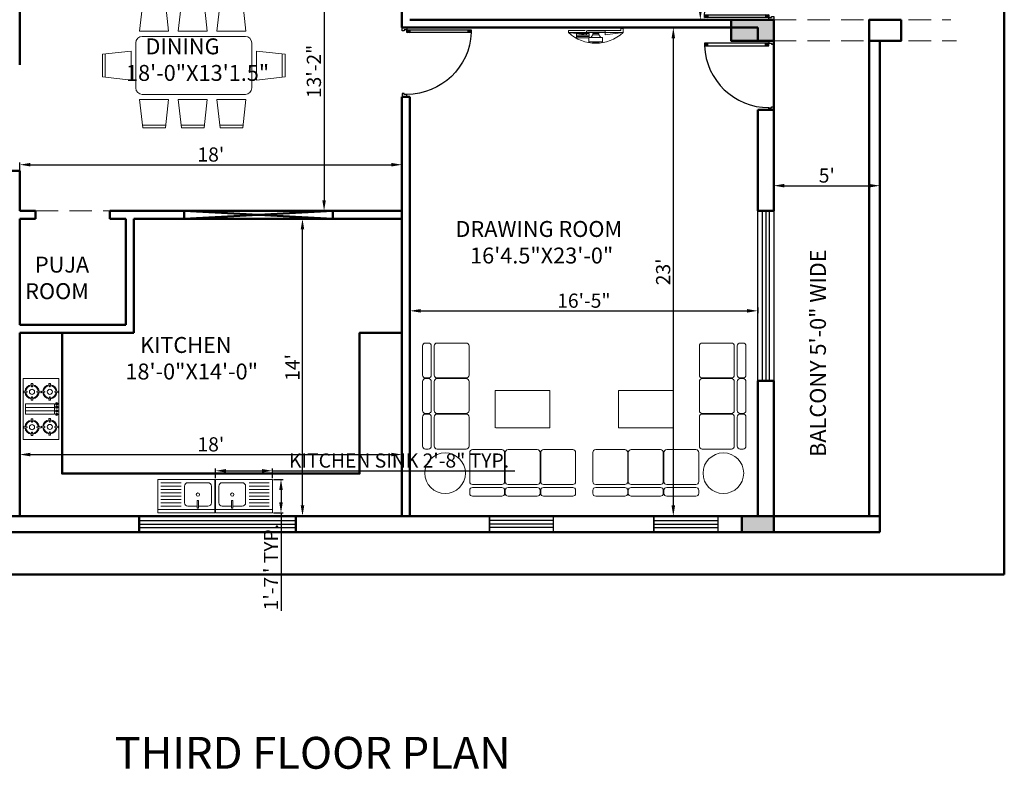
# Model space of a CAD drawing. Units: millimetres. Extents: x 1706 to 5913, y 156 to 1716.
# Tile 11 of 26: x 3523 to 4080, y 219 to 642. Entities that reach past the tile are written whole.
import ezdxf

# ---------------------------------------------------------------- set-up
doc = ezdxf.new("R2010")
doc.units = ezdxf.units.MM
doc.linetypes.add('DASHED', pattern=[19.05, 12.7, -6.35])
for name, color, linetype, lineweight in [('A-ANNO-DIMS', 2, 'Continuous', 18), ('A-ANNO-TEXT', 7, 'Continuous', 18), ('A-AREA-IDEN', 3, 'Continuous', 18), ('A-COLS', 20, 'Continuous', 50), ('A-DOOR', 4, 'Continuous', 25), ('A-FLOR-OVHD', 9, 'DASHED', 18), ('A-FURN', 8, 'Continuous', 18), ('A-GLAZ', 150, 'Continuous', 25), ('A-WALL', 7, 'Continuous', 50)]:
    doc.layers.add(name, color=color, linetype=linetype, lineweight=lineweight)
doc.styles.get("Standard").update_dxf_attribs({"font": 'arial.ttf'})
doc.dimstyles.new('ISO-25', dxfattribs={"dimtxt": 8, "dimasz": 6, "dimexe": 1.25, "dimexo": 0.625, "dimtad": 1, "dimdec": 0, "dimlunit": 3, "dimtxsty": 'Standard', "dimcen": 2.5, "dimadec": 0, "dimazin": 0, "dimtfac": 1, "dimtdec": 0, "dimtmove": 0, "dimatfit": 3, "dimfxl": 1, "dimarcsym": 0})

# ---------------------------------------------------------------- blocks, each defined once
blk = doc.blocks.new('Puerta 01')
for p, q in [((-0.775, -0.026), (-0.737, -0.058)), ((-0.775, -0.058), (-0.737, -0.026)), ((-0.737, -0.058), (-0.737, -0.026)), ((-0.028, -0.058), (-0.066, -0.026)), ((-0.028, -0.026), (-0.066, -0.058)), ((-0.066, -0.058), (-0.066, -0.026))]:
    blk.add_line(p, q)
for points in [[(-0.028, 0), (-0.028, -0.026), (0.004, -0.026), (0.004, -0.036), (0.028, -0.036), (0.028, 0)], [(-0.028, -0.026), (-0.775, -0.026), (-0.775, -0.058), (-0.028, -0.058)], [(0.004, -0.774), (0.004, -0.764), (0.028, -0.764), (0.028, -0.8), (-0.028, -0.8), (-0.028, -0.774)]]:
    blk.add_lwpolyline(points, close=True)
blk.add_arc((-0.028, -0.026), 0.747, 182.4545, 270)
blk = doc.blocks.new('A$C57CF26DA')
for p, q in [((0, 0), (0, 420)), ((720, 420), (0, 420)), ((167, 413), (147, 413)), ((147, 413), (152, 373)), ((152, 373), (162, 373)), ((162, 373), (167, 413)), ((300, 391), (300, 49)), ((300, 391), (420, 391)), ((340, 391), (340, 49)), ((380, 391), (380, 49)), ((420, 391), (420, 49)), ((584, 413), (564, 413)), ((564, 413), (569, 373)), ((569, 373), (579, 373)), ((579, 373), (584, 413)), ((720, 0), (720, 420)), ((99, 320), (59, 325)), ((59, 325), (59, 305)), ((59, 305), (99, 310)), ((99, 310), (99, 320)), ((152, 257), (147, 217)), ((162, 257), (152, 257)), ((167, 217), (162, 257)), ((255, 325), (215, 320)), ((215, 320), (215, 310)), ((215, 310), (255, 305)), ((255, 305), (255, 325)), ((516, 320), (476, 325)), ((476, 325), (476, 305)), ((476, 305), (516, 310)), ((516, 310), (516, 320)), ((569, 257), (564, 217)), ((579, 257), (569, 257)), ((584, 217), (579, 257)), ((672, 325), (632, 320)), ((632, 320), (632, 310)), ((632, 310), (672, 305)), ((672, 305), (672, 325)), ((147, 217), (167, 217)), ((167, 203), (147, 203)), ((147, 203), (152, 163)), ((152, 163), (162, 163)), ((162, 163), (167, 203)), ((581, 203), (561, 203)), ((561, 203), (566, 163)), ((564, 217), (584, 217)), ((566, 163), (576, 163)), ((576, 163), (581, 203)), ((99, 110), (59, 115)), ((59, 115), (59, 95)), ((59, 95), (99, 100)), ((99, 100), (99, 110)), ((152, 47), (147, 7)), ((147, 7), (167, 7)), ((162, 47), (152, 47)), ((167, 7), (162, 47)), ((255, 115), (215, 110)), ((215, 110), (215, 100)), ((215, 100), (255, 95)), ((255, 95), (255, 115)), ((302, 39), (295, 39)), ((295, 39), (295, 11)), ((295, 11), (302, 11)), ((420, 49), (300, 49)), ((302, 11), (302, 39)), ((341, 39), (334, 39)), ((334, 39), (334, 11)), ((334, 11), (341, 11)), ((341, 11), (341, 39)), ((380, 11), (380, 39)), ((380, 39), (386, 39)), ((386, 11), (380, 11)), ((386, 39), (386, 11)), ((419, 11), (419, 39)), ((419, 39), (426, 39)), ((426, 11), (419, 11)), ((426, 39), (426, 11)), ((513, 110), (473, 115)), ((473, 115), (473, 95)), ((473, 95), (513, 100)), ((513, 100), (513, 110)), ((566, 47), (561, 7)), ((561, 7), (581, 7)), ((576, 47), (566, 47)), ((581, 7), (576, 47)), ((669, 115), (629, 110)), ((629, 110), (629, 100)), ((629, 100), (669, 95)), ((669, 95), (669, 115)), ((720, 0), (0, 0))]:
    blk.add_line(p, q)
for centre in [(157, 315), (574, 315), (157, 105), (571, 105)]:
    blk.add_circle(centre, 30)
for centre, radius, start, end in [((157, 315), 83, 95.5849, 174.4151), ((157, 315), 73, 95.3738, 174.6262), ((157, 315), 73, 5.3738, 84.6262), ((157, 315), 83, 5.5849, 84.4151), ((574, 315), 83, 95.5849, 174.4151), ((574, 315), 73, 95.3738, 174.6262), ((574, 315), 73, 5.3738, 84.6262), ((574, 315), 83, 5.5849, 84.4151), ((157, 315), 83, 185.5849, 264.4151), ((157, 315), 73, 185.3738, 264.6262), ((157, 315), 73, 275.3738, 354.6262), ((157, 315), 83, 275.5849, 354.4151), ((574, 315), 83, 185.5849, 264.4151), ((574, 315), 73, 185.3738, 264.6262), ((574, 315), 73, 275.3738, 354.6262), ((574, 315), 83, 275.5849, 354.4151), ((157, 105), 83, 95.5849, 174.4151), ((157, 105), 73, 95.3738, 174.6262), ((157, 105), 73, 5.3738, 84.6262), ((157, 105), 83, 5.5849, 84.4151), ((571, 105), 83, 95.5849, 174.4151), ((571, 105), 73, 95.3738, 174.6262), ((571, 105), 73, 5.3738, 84.6262), ((571, 105), 83, 5.5849, 84.4151), ((157, 105), 83, 185.5849, 264.4151), ((157, 105), 73, 185.3738, 264.6262), ((157, 105), 73, 275.3738, 354.6262), ((157, 105), 83, 275.5849, 354.4151), ((298, 25), 13.7, 104.4775, 255.5225), ((298, 25), 13.7, 284.4775, 75.5225), ((337, 25), 13.7, 104.4775, 255.5225), ((337, 25), 13.7, 284.4775, 75.5225), ((383, 25), 13.7, 104.4775, 255.5225), ((383, 25), 13.7, 284.4775, 75.5225), ((422, 25), 13.7, 104.4775, 255.5225), ((422, 25), 13.7, 284.4775, 75.5225), ((571, 105), 83, 185.5849, 264.4151), ((571, 105), 73, 185.3738, 264.6262), ((571, 105), 73, 275.3738, 354.6262), ((571, 105), 83, 275.5849, 354.4151)]:
    blk.add_arc(centre, radius, start, end)
blk = doc.blocks.new('A$C3404121D')
for p, q in [((0, 0), (0, 500)), ((0, 500), (850, 500)), ((0, 450), (850, 450)), ((850, 500), (850, 0)), ((50, 100), (50, 350)), ((100, 400), (240, 400)), ((240, 431), (240, 425)), ((260, 431), (240, 431)), ((240, 425), (240, 315)), ((240, 315), (260, 315)), ((260, 431), (260, 315)), ((260, 400), (400, 400)), ((450, 100), (450, 350)), ((502, 400), (801, 400)), ((502, 350), (801, 350)), ((502, 300), (801, 300)), ((502, 250), (801, 250)), ((502, 200), (801, 200)), ((502, 150), (801, 150)), ((850, 0), (0, 0)), ((400, 50), (100, 50)), ((502, 100), (801, 100)), ((801, 50), (502, 50))]:
    blk.add_line(p, q)
blk.add_circle((250, 228), 25)
for centre, start, end in [((100, 350), 90, 180), ((400, 350), 0, 90), ((100, 100), 180, 270), ((400, 100), 270, 0)]:
    blk.add_arc(centre, 50, start, end)
blk = doc.blocks.new('A$C59D7588A')
for p, q in [((0.575, 1.5), (0.623, 1.943)), ((0.618, 1.9), (0.982, 1.9)), ((0.623, 1.943), (0.978, 1.943)), ((0.978, 1.943), (1.025, 1.5)), ((1.175, 1.5), (1.223, 1.943)), ((1.218, 1.9), (1.582, 1.9)), ((1.223, 1.943), (1.578, 1.943)), ((1.578, 1.943), (1.625, 1.5)), ((1.775, 1.5), (1.823, 1.943)), ((1.818, 1.9), (2.182, 1.9)), ((1.823, 1.943), (2.178, 1.943)), ((2.178, 1.943), (2.225, 1.5)), ((1.025, 1.5), (0.575, 1.5)), ((0.616, 1.421), (2.216, 1.421)), ((1.625, 1.5), (1.175, 1.5)), ((2.225, 1.5), (1.775, 1.5)), ((0.516, 0.621), (0.516, 1.321)), ((2.316, 1.321), (2.316, 0.621)), ((0, 1.146), (0.443, 1.194)), ((0, 0.792), (0, 1.146)), ((0.043, 0.787), (0.043, 1.151)), ((0.443, 1.194), (0.443, 0.744)), ((2.832, 1.146), (2.389, 1.194)), ((2.389, 1.194), (2.389, 0.744)), ((2.789, 0.787), (2.789, 1.151)), ((2.832, 0.792), (2.832, 1.146)), ((0.443, 0.744), (0, 0.792)), ((2.389, 0.744), (2.832, 0.792)), ((2.216, 0.521), (0.616, 0.521)), ((1.025, 0.443), (0.575, 0.443)), ((0.575, 0.443), (0.623, 0)), ((0.978, 0), (1.025, 0.443)), ((1.625, 0.443), (1.175, 0.443)), ((1.175, 0.443), (1.223, 0)), ((1.578, 0), (1.625, 0.443)), ((2.225, 0.443), (1.775, 0.443)), ((1.775, 0.443), (1.823, 0)), ((2.178, 0), (2.225, 0.443)), ((0.618, 0.043), (0.982, 0.043)), ((1.218, 0.043), (1.582, 0.043)), ((1.818, 0.043), (2.182, 0.043)), ((0.623, 0), (0.978, 0)), ((1.223, 0), (1.578, 0)), ((1.823, 0), (2.178, 0))]:
    blk.add_line(p, q)
for centre, start, end in [((0.616, 1.321), 90, 180), ((2.216, 1.321), 0, 90), ((0.616, 0.621), 180, 270), ((2.216, 0.621), 270, 0)]:
    blk.add_arc(centre, 0.1, start, end)
blk = doc.blocks.new('A$C753D6792')
at = {"linetype": 'ByBlock'}
for p, q in [((0, 2530), (0, 2580)), ((50, 2630), (550, 2630)), ((600, 2580), (600, 2530)), ((610, 2530), (610, 2580)), ((660, 2630), (1160, 2630)), ((1210, 2580), (1210, 2530)), ((1220, 2530), (1220, 2580)), ((1270, 2630), (1770, 2630)), ((1820, 2580), (1820, 2530)), ((0, 1880), (0, 2380)), ((550, 2480), (50, 2480)), ((550, 2430), (50, 2430)), ((600, 2380), (600, 1880)), ((610, 1880), (610, 2380)), ((1160, 2480), (660, 2480)), ((1160, 2430), (660, 2430)), ((1210, 2380), (1210, 1880)), ((1220, 1880), (1220, 2380)), ((1770, 2480), (1270, 2480)), ((1770, 2430), (1270, 2430)), ((1820, 1880), (1820, 2380)), ((50, 1830), (427, 1830)), ((387, 1830), (550, 1830)), ((660, 1830), (1037, 1830)), ((997, 1830), (1160, 1830)), ((1270, 1830), (1647, 1830)), ((1607, 1830), (1770, 1830)), ((1830, 1770), (1830, 1393)), ((1880, 1820), (2380, 1820)), ((2430, 1270), (2430, 1770)), ((2480, 1270), (2480, 1770)), ((2530, 1820), (2580, 1820)), ((2630, 1770), (2630, 1270)), ((442, 815), (442, 1455)), ((442, 1455), (1372, 1455)), ((1382, 1455), (1382, 815)), ((1830, 1433), (1830, 1270)), ((2380, 1220), (1880, 1220)), ((1880, 1210), (2380, 1210)), ((2580, 1220), (2530, 1220)), ((2530, 1210), (2580, 1210)), ((1830, 1160), (1830, 783)), ((2430, 660), (2430, 1160)), ((2480, 660), (2480, 1160)), ((2630, 1160), (2630, 660)), ((1382, 815), (442, 815)), ((1830, 823), (1830, 660)), ((1830, 550), (1830, 173)), ((2380, 610), (1880, 610)), ((1880, 600), (2380, 600)), ((2430, 50), (2430, 550)), ((2480, 50), (2480, 550)), ((2580, 610), (2530, 610)), ((2530, 600), (2580, 600)), ((2630, 550), (2630, 50)), ((1830, 213), (1830, 50)), ((2380, 0), (1880, 0)), ((2580, 0), (2530, 0))]:
    blk.add_line(p, q, dxfattribs=at)
blk.add_circle((2242, 2235), 349, dxfattribs=at)
for centre, start, end in [((50, 2580), 90, 180), ((550, 2580), 0, 90), ((550, 2580), 0, 90), ((660, 2580), 90, 180), ((1160, 2580), 0, 90), ((1160, 2580), 0, 90), ((1270, 2580), 90, 180), ((1770, 2580), 0, 90), ((1770, 2580), 0, 90), ((50, 2530), 180, 270), ((50, 2380), 90, 180), ((550, 2530), 270, 0), ((550, 2530), 270, 0), ((550, 2380), 0, 90), ((550, 2380), 0, 90), ((660, 2530), 180, 270), ((660, 2380), 90, 180), ((1160, 2530), 270, 0), ((1160, 2530), 270, 0), ((1160, 2380), 0, 90), ((1160, 2380), 0, 90), ((1270, 2530), 180, 270), ((1270, 2380), 90, 180), ((1770, 2530), 270, 0), ((1770, 2530), 270, 0), ((1770, 2380), 0, 90), ((1770, 2380), 0, 90), ((50, 1880), 180, 270), ((550, 1880), 270, 0), ((660, 1880), 180, 270), ((1160, 1880), 270, 0), ((1270, 1880), 180, 270), ((1770, 1880), 270, 0), ((1880, 1770), 90, 180), ((2380, 1770), 0, 90), ((2530, 1770), 90, 180), ((2580, 1770), 0, 90), ((1880, 1270), 180, 270), ((1880, 1160), 90, 180), ((2380, 1270), 270, 0), ((2380, 1270), 270, 0), ((2380, 1160), 0, 90), ((2530, 1270), 180, 270), ((2530, 1270), 180, 270), ((2530, 1160), 90, 180), ((2580, 1270), 270, 0), ((2580, 1270), 270, 0), ((2580, 1160), 0, 90), ((1880, 660), 180, 270), ((1880, 550), 90, 180), ((2380, 660), 270, 0), ((2380, 660), 270, 0), ((2380, 550), 0, 90), ((2530, 660), 180, 270), ((2530, 660), 180, 270), ((2530, 550), 90, 180), ((2580, 660), 270, 0), ((2580, 660), 270, 0), ((2580, 550), 0, 90), ((1880, 50), 180, 270), ((2380, 50), 270, 0), ((2380, 50), 270, 0), ((2530, 50), 180, 270), ((2530, 50), 180, 270), ((2580, 50), 270, 0), ((2580, 50), 270, 0)]:
    blk.add_arc(centre, 50, start, end, dxfattribs=at)
blk = doc.blocks.new('tv unit')
for p, q in [((4607, 2403), (5207, 2403)), ((4607, 2203), (4607, 2403)), ((5853, 2588), (5205, 2588)), ((5205, 2392), (5205, 2588)), ((5853, 2392), (5205, 2392)), ((5207, 2403), (5207, 2203)), ((5293, 2392), (5385, 2268)), ((5765, 2392), (5672, 2268)), ((5853, 2392), (5853, 2588)), ((5079, 2257), (4229, 2157)), ((6829, 2157), (4229, 2157)), ((4229, 2157), (4229, 2057)), ((5029, 2057), (4229, 2057)), ((4607, 2337), (5207, 2337)), ((4607, 2269), (5207, 2269)), ((5207, 2203), (4607, 2203)), ((5079, 2077), (5079, 2257)), ((5979, 2077), (5079, 2077)), ((6729, 2057), (5129, 2057)), ((5385, 2268), (5672, 2268)), ((5385, 2268), (5385, 2204)), ((5385, 2204), (5672, 2204)), ((5672, 2268), (5672, 2204)), ((5979, 2257), (6829, 2157)), ((5979, 2077), (5979, 2257)), ((6729, 2057), (6729, 1957)), ((6829, 1957), (6729, 1957)), ((6829, 2157), (6829, 1957))]:
    blk.add_line(p, q)
for points in [[(6829, 2157, 0.386509), (4229, 2157, -2.260033)], [(4242, 2140, -0.414214), (4270, 2168), (4561, 2168)]]:
    blk.add_lwpolyline(points, format="xyb")
blk.add_arc((5529, 609), 2006, 80.6925, 99.3075)
blk = doc.blocks.new('*D159')
at = {"layer": 'A-ANNO-DIMS', "color": 0, "lineweight": -2, "transparency": 16777216}
for p, q in [((3907.19, 843.39), (3906.51, 843.39)), ((3907.76, 837.39), (3907.76, 648.39)), ((3907.19, 642.39), (3906.51, 642.39))]:
    blk.add_line(p, q, dxfattribs=at)
at = {"layer": 'A-ANNO-DIMS', "color": 0, "transparency": 16777216}
for points in [[(3906.76, 837.39), (3908.76, 837.39), (3907.76, 843.39)], [(3906.76, 648.39), (3908.76, 648.39), (3907.76, 642.39)]]:
    blk.add_solid(points, dxfattribs=at)
at = {"layer": 'Defpoints', "color": 0, "transparency": 16777216}
for p in [(3907.82, 843.39), (3907.76, 642.39), (3907.82, 642.39)]:
    blk.add_point(p, dxfattribs=at)
at = {"layer": 'A-ANNO-DIMS', "color": 0, "transparency": 16777216, "insert": (3903.05, 742.89), "char_height": 8, "attachment_point": 5, "rotation": 90}
blk.add_mtext('16\'-9"', dxfattribs=at)
blk = doc.blocks.new('*D161')
at = {"layer": 'A-ANNO-DIMS', "color": 0, "lineweight": -2, "transparency": 16777216}
for p, q in [((3692.59, 691.89), (3696.44, 691.89)), ((3695.19, 685.89), (3695.19, 540.39)), ((3692.59, 534.39), (3696.44, 534.39))]:
    blk.add_line(p, q, dxfattribs=at)
at = {"layer": 'A-ANNO-DIMS', "color": 0, "transparency": 16777216}
for points in [[(3694.19, 685.89), (3696.19, 685.89), (3695.19, 691.89)], [(3694.19, 540.39), (3696.19, 540.39), (3695.19, 534.39)]]:
    blk.add_solid(points, dxfattribs=at)
at = {"layer": 'Defpoints', "color": 0, "transparency": 16777216}
for p in [(3691.96, 691.89), (3691.96, 534.39), (3695.19, 534.39)]:
    blk.add_point(p, dxfattribs=at)
at = {"layer": 'A-ANNO-DIMS', "color": 0, "transparency": 16777216, "insert": (3690.48, 613.14), "char_height": 8, "attachment_point": 5, "rotation": 90}
blk.add_mtext('13\'-2"', dxfattribs=at)
blk = doc.blocks.new('*D162')
at = {"layer": 'A-ANNO-DIMS', "color": 0, "lineweight": -2, "transparency": 16777216}
for p, q in [((3523.21, 548.14), (3523.21, 561.7)), ((3529.21, 560.45), (3733.21, 560.45)), ((3739.21, 548.14), (3739.21, 561.7))]:
    blk.add_line(p, q, dxfattribs=at)
at = {"layer": 'A-ANNO-DIMS', "color": 0, "transparency": 16777216}
for points in [[(3529.21, 561.45), (3529.21, 559.45), (3523.21, 560.45)], [(3733.21, 561.45), (3733.21, 559.45), (3739.21, 560.45)]]:
    blk.add_solid(points, dxfattribs=at)
at = {"layer": 'Defpoints', "color": 0, "transparency": 16777216}
for p in [(3739.21, 560.45), (3523.21, 547.51), (3739.21, 547.51)]:
    blk.add_point(p, dxfattribs=at)
at = {"layer": 'A-ANNO-DIMS', "color": 0, "transparency": 16777216, "insert": (3631.21, 565.16), "char_height": 8, "attachment_point": 5}
blk.add_mtext("18'", dxfattribs=at)
blk = doc.blocks.new('*D163')
at = {"layer": 'A-ANNO-DIMS', "color": 0, "lineweight": -2, "transparency": 16777216}
for p, q in [((3683.98, 529.89), (3681.74, 529.89)), ((3682.99, 367.89), (3682.99, 523.89)), ((3683.98, 361.89), (3681.74, 361.89))]:
    blk.add_line(p, q, dxfattribs=at)
at = {"layer": 'A-ANNO-DIMS', "color": 0, "transparency": 16777216}
for points in [[(3681.99, 523.89), (3683.99, 523.89), (3682.99, 529.89)], [(3681.99, 367.89), (3683.99, 367.89), (3682.99, 361.89)]]:
    blk.add_solid(points, dxfattribs=at)
at = {"layer": 'Defpoints', "color": 0, "transparency": 16777216}
for p in [(3682.99, 529.89), (3684.6, 529.89), (3684.6, 361.89)]:
    blk.add_point(p, dxfattribs=at)
at = {"layer": 'A-ANNO-DIMS', "color": 0, "transparency": 16777216, "insert": (3678.34, 445.89), "char_height": 8, "attachment_point": 5, "rotation": 90}
blk.add_mtext("14'", dxfattribs=at)
blk = doc.blocks.new('*D164')
at = {"layer": 'A-ANNO-DIMS', "color": 0, "lineweight": -2, "transparency": 16777216}
for p, q in [((3523.21, 389.35), (3523.21, 397.93)), ((3529.21, 396.68), (3733.21, 396.68)), ((3739.21, 389.35), (3739.21, 397.93))]:
    blk.add_line(p, q, dxfattribs=at)
at = {"layer": 'A-ANNO-DIMS', "color": 0, "transparency": 16777216}
for points in [[(3529.21, 397.68), (3529.21, 395.68), (3523.21, 396.68)], [(3733.21, 397.68), (3733.21, 395.68), (3739.21, 396.68)]]:
    blk.add_solid(points, dxfattribs=at)
at = {"layer": 'Defpoints', "color": 0, "transparency": 16777216}
for p in [(3739.21, 396.68), (3523.21, 388.72), (3739.21, 388.72)]:
    blk.add_point(p, dxfattribs=at)
at = {"layer": 'A-ANNO-DIMS', "color": 0, "transparency": 16777216, "insert": (3631.21, 401.39), "char_height": 8, "attachment_point": 5}
blk.add_mtext("18'", dxfattribs=at)
blk = doc.blocks.new('*D165')
at = {"layer": 'A-ANNO-DIMS', "color": 0, "lineweight": -2, "transparency": 16777216}
for p, q in [((3889.02, 637.89), (3893.75, 637.89)), ((3892.5, 631.89), (3892.5, 367.89)), ((3889.02, 361.89), (3893.75, 361.89))]:
    blk.add_line(p, q, dxfattribs=at)
at = {"layer": 'A-ANNO-DIMS', "color": 0, "transparency": 16777216}
for points in [[(3891.5, 631.89), (3893.5, 631.89), (3892.5, 637.89)], [(3891.5, 367.89), (3893.5, 367.89), (3892.5, 361.89)]]:
    blk.add_solid(points, dxfattribs=at)
at = {"layer": 'Defpoints', "color": 0, "transparency": 16777216}
for p in [(3888.39, 637.89), (3888.39, 361.89), (3892.5, 361.89)]:
    blk.add_point(p, dxfattribs=at)
at = {"layer": 'A-ANNO-DIMS', "color": 0, "transparency": 16777216, "insert": (3887.78, 499.89), "char_height": 8, "attachment_point": 5, "rotation": 90}
blk.add_mtext("23'", dxfattribs=at)
blk = doc.blocks.new('*D166')
at = {"layer": 'A-ANNO-DIMS', "color": 0, "lineweight": -2, "transparency": 16777216}
for p, q in [((3743.71, 479.76), (3743.71, 476.62)), ((3940.21, 479.76), (3940.21, 476.62)), ((3749.71, 477.87), (3934.21, 477.87))]:
    blk.add_line(p, q, dxfattribs=at)
at = {"layer": 'A-ANNO-DIMS', "color": 0, "transparency": 16777216}
for points in [[(3749.71, 478.87), (3749.71, 476.87), (3743.71, 477.87)], [(3934.21, 478.87), (3934.21, 476.87), (3940.21, 477.87)]]:
    blk.add_solid(points, dxfattribs=at)
at = {"layer": 'Defpoints', "color": 0, "transparency": 16777216}
for p in [(3743.71, 480.39), (3940.21, 480.39), (3940.21, 477.87)]:
    blk.add_point(p, dxfattribs=at)
at = {"layer": 'A-ANNO-DIMS', "color": 0, "transparency": 16777216, "insert": (3841.96, 482.58), "char_height": 8, "attachment_point": 5}
blk.add_mtext('16\'-5"', dxfattribs=at)
blk = doc.blocks.new('*D168')
at = {"layer": 'A-ANNO-DIMS', "color": 0, "lineweight": -2, "transparency": 16777216}
for p, q in [((3949.21, 549.96), (3949.21, 547.34)), ((3955.21, 548.59), (4003.21, 548.59)), ((4009.21, 549.96), (4009.21, 547.34))]:
    blk.add_line(p, q, dxfattribs=at)
at = {"layer": 'A-ANNO-DIMS', "color": 0, "transparency": 16777216}
for points in [[(3955.21, 549.59), (3955.21, 547.59), (3949.21, 548.59)], [(4003.21, 549.59), (4003.21, 547.59), (4009.21, 548.59)]]:
    blk.add_solid(points, dxfattribs=at)
at = {"layer": 'Defpoints', "color": 0, "transparency": 16777216}
for p in [(3949.21, 550.58), (4009.21, 550.58), (4009.21, 548.59)]:
    blk.add_point(p, dxfattribs=at)
at = {"layer": 'A-ANNO-DIMS', "color": 0, "transparency": 16777216, "insert": (3979.21, 553.29), "char_height": 8, "attachment_point": 5}
blk.add_mtext("5'", dxfattribs=at)
blk = doc.blocks.new('*D221')
at = {"layer": 'A-ANNO-DIMS', "color": 0, "lineweight": -2, "transparency": 16777216}
for p, q in [((3633.81, 383.28), (3633.81, 388.74)), ((3639.81, 387.49), (3660.02, 387.49)), ((3666.02, 383.28), (3666.02, 388.74)), ((3666.02, 387.49), (3803.03, 387.49))]:
    blk.add_line(p, q, dxfattribs=at)
at = {"layer": 'A-ANNO-DIMS', "color": 0, "transparency": 16777216}
for points in [[(3639.81, 388.49), (3639.81, 386.49), (3633.81, 387.49)], [(3660.02, 388.49), (3660.02, 386.49), (3666.02, 387.49)]]:
    blk.add_solid(points, dxfattribs=at)
at = {"layer": 'Defpoints', "color": 0, "transparency": 16777216}
for p in [(3666.02, 387.49), (3633.81, 382.65), (3666.02, 382.65)]:
    blk.add_point(p, dxfattribs=at)
at = {"layer": 'A-ANNO-DIMS', "color": 0, "transparency": 16777216, "insert": (3737.52, 392.25), "char_height": 8, "attachment_point": 5}
blk.add_mtext('KITCHEN SINK 2\'-8" TYP.', dxfattribs=at)
blk = doc.blocks.new('*D222')
at = {"layer": 'A-ANNO-DIMS', "color": 0, "lineweight": -2, "transparency": 16777216}
for p, q in [((3666.64, 382.65), (3672.1, 382.65)), ((3670.85, 376.65), (3670.85, 369.7)), ((3666.64, 363.7), (3672.1, 363.7)), ((3670.85, 363.7), (3670.85, 308.44))]:
    blk.add_line(p, q, dxfattribs=at)
at = {"layer": 'A-ANNO-DIMS', "color": 0, "transparency": 16777216}
for points in [[(3669.85, 376.65), (3671.85, 376.65), (3670.85, 382.65)], [(3669.85, 369.7), (3671.85, 369.7), (3670.85, 363.7)]]:
    blk.add_solid(points, dxfattribs=at)
at = {"layer": 'Defpoints', "color": 0, "transparency": 16777216}
for p in [(3666.02, 382.65), (3666.02, 363.7), (3670.85, 363.7)]:
    blk.add_point(p, dxfattribs=at)
at = {"layer": 'A-ANNO-DIMS', "color": 0, "transparency": 16777216, "insert": (3666.21, 333.07), "char_height": 8, "attachment_point": 5, "rotation": 90}
blk.add_mtext('1\'-7" TYP.', dxfattribs=at)

msp = doc.modelspace()

# ---------------------------------------------------------------- hatches: boundary and pattern name
at = {"layer": 'A-COLS'}
h = msp.add_hatch(color=256, dxfattribs=at)
h.dxf.hatch_style = 1
h.paths.add_polyline_path([(3949.21, 642.39), (3925.21, 642.39), (3925.21, 630.39), (3949.21, 630.39)])
h = msp.add_hatch(color=256, dxfattribs=at)
h.dxf.hatch_style = 1
h.paths.add_polyline_path([(3949.21, 361.89), (3931.21, 361.89), (3931.21, 352.89), (3949.21, 352.89)])

# ---------------------------------------------------------------- linework, layer by layer
msp.add_lwpolyline([(3925.21, 642.39), (3949.21, 642.39), (3949.21, 630.39), (3925.21, 630.39)], close=True, dxfattribs=at)
msp.add_lwpolyline([(3949.43, 361.89), (3931.21, 361.89), (3931.21, 352.89), (3949.21, 352.89), (3949.21, 361.89)], dxfattribs=at)
at = {"layer": 'A-FLOR-OVHD'}
for p, q in [((3949.21, 642.39), (4049.33, 642.39)), ((3949.21, 630.39), (4052.51, 630.39)), ((3532.21, 534.39), (3574.21, 534.39))]:
    msp.add_line(p, q, dxfattribs=at)
at = {"layer": 'A-GLAZ'}
for p, q in [((3942.71, 534.39), (3942.71, 438.39)), ((3944.71, 534.39), (3944.71, 438.39)), ((3946.71, 534.39), (3946.71, 438.39)), ((3788.58, 361.89), (3788.58, 352.89)), ((3824.58, 361.89), (3824.58, 352.89)), ((3881.58, 361.89), (3881.58, 352.89)), ((3917.58, 361.89), (3917.58, 352.89)), ((3590.71, 359.39), (3679.21, 359.39)), ((3590.71, 357.39), (3679.21, 357.39)), ((3824.58, 359.39), (3788.58, 359.39)), ((3824.58, 357.39), (3788.58, 357.39)), ((3881.58, 359.39), (3917.58, 359.39)), ((3881.58, 357.39), (3917.58, 357.39)), ((3590.71, 355.39), (3679.21, 355.39)), ((3824.58, 355.39), (3788.58, 355.39)), ((3881.58, 355.39), (3917.58, 355.39))]:
    msp.add_line(p, q, dxfattribs=at)
for points in [[(3940.21, 534.39), (3949.21, 534.39), (3949.21, 438.39), (3940.21, 438.39)], [(3590.71, 361.89), (3679.21, 361.89), (3679.21, 352.89), (3590.71, 352.89)], [(3788.58, 361.89), (3824.58, 361.89), (3824.58, 352.89), (3788.58, 352.89)], [(3881.58, 361.89), (3917.58, 361.89), (3917.58, 352.89), (3881.58, 352.89)]]:
    msp.add_lwpolyline(points, close=True, dxfattribs=at)
at = {"layer": 'A-WALL'}
for p, q in [((4079.51, 852.39), (4079.51, 328.89)), ((3523.21, 691.89), (3523.21, 616.89)), ((3739.21, 649.89), (3739.21, 637.89)), ((3743.71, 642.39), (3949.21, 642.39)), ((3949.21, 642.39), (3949.21, 630.39)), ((3739.21, 637.89), (3940.21, 637.89)), ((3940.21, 637.89), (3940.21, 630.39)), ((3949.21, 630.39), (3940.21, 630.39)), ((3949.21, 630.39), (3949.21, 591.39)), ((4003.21, 630.39), (4003.21, 361.89)), ((4009.21, 630.39), (4009.21, 361.89)), ((3739.21, 598.89), (3739.21, 361.89)), ((3739.21, 598.89), (3743.71, 598.89)), ((3743.71, 598.89), (3743.71, 361.89)), ((3940.21, 591.39), (3940.21, 534.39)), ((3949.21, 591.39), (3940.21, 591.39)), ((3949.21, 591.39), (3949.21, 534.39)), ((3518.71, 556.89), (3523.21, 556.89)), ((3523.21, 556.89), (3523.21, 534.39)), ((3523.21, 534.39), (3532.21, 534.39)), ((3532.21, 534.39), (3532.21, 529.89)), ((3574.21, 534.39), (3574.21, 529.89)), ((3574.21, 534.39), (3616.21, 534.39)), ((3616.21, 534.39), (3616.21, 529.89)), ((3700.21, 534.39), (3616.21, 529.89)), ((3616.21, 534.39), (3700.21, 529.89)), ((3700.21, 534.39), (3700.21, 529.89)), ((3700.21, 534.39), (3739.21, 534.39)), ((3949.21, 534.39), (3940.21, 534.39)), ((3523.21, 529.89), (3523.21, 469.89)), ((3523.21, 529.89), (3532.21, 529.89)), ((3574.21, 529.89), (3583.21, 529.89)), ((3583.21, 529.89), (3583.21, 469.89)), ((3587.71, 529.89), (3587.71, 465.39)), ((3587.71, 529.89), (3616.21, 529.89)), ((3700.21, 529.89), (3739.21, 529.89)), ((3523.21, 469.89), (3583.21, 469.89)), ((3523.21, 465.39), (3523.21, 361.89)), ((3523.21, 465.39), (3587.71, 465.39)), ((3940.21, 438.39), (3940.21, 361.89)), ((3949.21, 438.39), (3940.21, 438.39)), ((3949.21, 438.39), (3949.21, 361.89)), ((3214.21, 361.89), (4009.21, 361.89)), ((3590.71, 361.89), (3590.71, 352.89)), ((3679.21, 361.89), (3679.21, 352.89)), ((3949.21, 361.89), (3949.21, 352.89)), ((3949.21, 352.89), (3949.21, 361.89)), ((4009.21, 361.89), (4009.21, 352.89)), ((3209.71, 352.89), (4009.21, 352.89)), ((3184.21, 328.89), (4079.51, 328.89))]:
    msp.add_line(p, q, dxfattribs=at)
for points in [[(4021.21, 642.39), (4003.21, 642.39), (4003.21, 630.39), (4021.21, 630.39)], [(3616.21, 534.39), (3700.21, 534.39), (3700.21, 529.89), (3616.21, 529.89)]]:
    msp.add_lwpolyline(points, close=True, dxfattribs=at)
msp.add_lwpolyline([(3547.21, 465.39), (3547.21, 385.89), (3715.21, 385.89), (3715.21, 465.39), (3739.21, 465.39)], dxfattribs=at)

# ---------------------------------------------------------------- block references
at = {"layer": 'A-DOOR', "xscale": -48.75000000000287, "yscale": 48.75000000000287, "zscale": 48.75000000000287, "rotation": 180}
msp.add_blockref('Puerta 01', (3947.85, 642.39), dxfattribs=at)
at = {"layer": 'A-DOOR', "yscale": 48.75000000000287, "zscale": 48.75000000000287}
for p, xscale in [((3740.58, 637.89), -48.75000000000287), ((3947.85, 630.39), 48.75000000000287)]:
    msp.add_blockref('Puerta 01', p, dxfattribs=dict(at, xscale=xscale))
at = {"layer": 'A-FURN', "xscale": 36.4071025162376, "yscale": 36.4071025162376, "zscale": 36.4071025162376}
msp.add_blockref('A$C59D7588A', (3570.02, 581.2), dxfattribs=at)
at = {"layer": 'A-FURN'}
for name, p, xscale, yscale, zscale, rotation in [('tv unit', (3783.17, 660.62), -0.0118512648876472, 0.0118512648876472, 0.0118512648876472, 180), ('A$C753D6792', (3837.33, 459.67), 0.0329035460231199, 0.0329035460231199, 0.0329035460231199, 180), ('A$C753D6792', (3847.01, 459.67), -0.0329035460231199, 0.0329035460231199, 0.0329035460231199, 180), ('A$C57CF26DA', (3545.25, 439.61), -0.0478777176975714, 0.0478777176975714, 0.0478777176975714, 90), ('A$C3404121D', (3633.39, 382.65), 0.0378984485580132, 0.0378984485580132, 0.0378984485580132, 180), ('A$C3404121D', (3633.81, 382.65), -0.0378984485580132, 0.0378984485580132, 0.0378984485580132, 180)]:
    msp.add_blockref(name, p, dxfattribs=dict(at, xscale=xscale, yscale=yscale, zscale=zscale, rotation=rotation))

# ---------------------------------------------------------------- texts
at = {"layer": 'A-ANNO-TEXT', "insert": (3576.87, 237.14), "char_height": 18, "attachment_point": 1}
msp.add_mtext_dynamic_manual_height_columns('THIRD FLOOR PLAN', width=352.5721, gutter_width=12.5, heights=[0], dxfattribs=at)
at = {"layer": 'A-AREA-IDEN', "char_height": 9, "attachment_point": 1}
for s, width, insert in [('    DINING\\P18\'-0"X13\'1.5"', 67.9131, (3583.28, 631.82)), ('    DRAWING ROOM\\P       16\'4.5"X23\'-0"', 125.2434, (3758.42, 528.63)), ('  PUJA ROOM', 67.9131, (3526.31, 508.49)), ('    KITCHEN\\P 18\'-0"X14\'-0"', 99.443, (3580.17, 463.09))]:
    msp.add_mtext_dynamic_manual_height_columns(s, width=width, gutter_width=12.5, heights=[0], dxfattribs=dict(at, insert=insert))
at = {"layer": 'A-AREA-IDEN', "insert": (3969.71, 384.32), "char_height": 9, "attachment_point": 1, "rotation": 90}
msp.add_mtext_dynamic_manual_height_columns('    BALCONY 5\'-0" WIDE', width=166.3136, gutter_width=12.5, heights=[0], dxfattribs=at)

# ---------------------------------------------------------------- dimensions: what is measured, and where the dimension line sits
at = {"layer": 'A-ANNO-DIMS'}
for base, p1, p2, picture, middle in [((3907.76, 642.39), (3907.82, 843.39), (3907.82, 642.39), '*D159', (3903.05, 742.89)), ((3695.18861206, 534.38567161), (3691.96347462, 691.88567161), (3691.96347462, 534.38567161), '*D161', (3690.47629964, 613.13567161)), ((3892.5, 361.89), (3888.39, 637.89), (3888.39, 361.89), '*D165', (3887.78, 499.89)), ((3682.99, 529.89), (3684.6, 361.89), (3684.6, 529.89), '*D163', (3678.34, 445.89))]:
    dim = msp.add_linear_dim(base=base, p1=p1, p2=p2, angle=90, dimstyle='ISO-25', override={"dimclrd": 0, "dimclre": 0, "dimclrt": 0}, dxfattribs=at)
    dim.commit()
    dim.dimension.update_dxf_attribs({"geometry": picture, "text_midpoint": middle})
for base, p1, p2, picture, middle in [((3739.21, 560.45), (3523.21, 547.51), (3739.21, 547.51), '*D162', (3631.21, 565.16)), ((4009.21, 548.59), (3949.21, 550.58), (4009.21, 550.58), '*D168', (3979.21, 553.29)), ((3940.21347462, 477.86812213), (3743.71347462, 480.38567161), (3940.21347462, 480.38567161), '*D166', (3841.96347462, 482.57770603)), ((3739.21, 396.68), (3523.21, 388.72), (3739.21, 388.72), '*D164', (3631.21, 401.39))]:
    dim = msp.add_linear_dim(base=base, p1=p1, p2=p2, dimstyle='ISO-25', override={"dimclrd": 0, "dimclre": 0, "dimclrt": 0}, dxfattribs=at)
    dim.commit()
    dim.dimension.update_dxf_attribs({"geometry": picture, "text_midpoint": middle})
dim = msp.add_linear_dim(base=(3666.02, 387.49), p1=(3633.81, 382.65), p2=(3666.02, 382.65), text='KITCHEN SINK <> TYP.', dimstyle='ISO-25', override={"dimdec": 1, "dimrnd": 0, "dimzin": 1, "dimlunit": 4, "dimfrac": 2}, dxfattribs=at)
dim.commit()
dim.dimension.update_dxf_attribs({"geometry": '*D221', "text_midpoint": (3737.52, 392.25)})
dim = msp.add_linear_dim(base=(3670.8515, 363.7043), p1=(3666.0194, 382.6535), p2=(3666.0194, 363.7043), angle=270, text='<> TYP.', dimstyle='ISO-25', override={"dimdec": 1, "dimrnd": 0, "dimzin": 1, "dimlunit": 4, "dimfrac": 2}, dxfattribs=at)
dim.commit()
dim.dimension.update_dxf_attribs({"geometry": '*D222', "text_midpoint": (3666.2074, 333.0738)})

doc.saveas('drawing.dxf')
